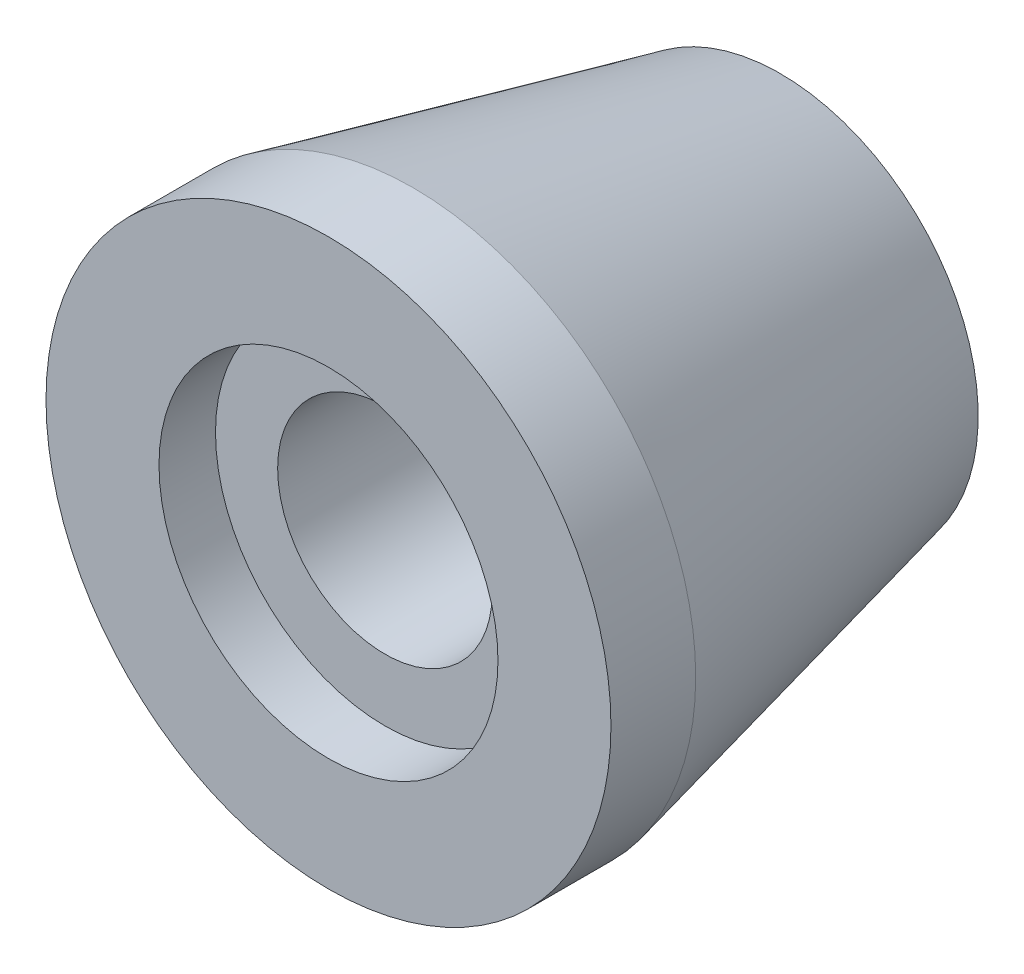
ISO-10303-21;
HEADER;
FILE_DESCRIPTION(('STEP AP214'),'2;1');
FILE_NAME('part.step','',(''),(''),'','','');
FILE_SCHEMA(('AUTOMOTIVE_DESIGN { 1 0 10303 214 1 1 1 1 }'));
ENDSEC;
DATA;
#1=APPLICATION_CONTEXT('core data for automotive mechanical design processes');
#2=APPLICATION_PROTOCOL_DEFINITION('international standard','automotive_design',2000,#1);
#3=PRODUCT_CONTEXT('',#1,'mechanical');
#4=PRODUCT('Part','Part','',(#3));
#5=PRODUCT_RELATED_PRODUCT_CATEGORY('part','',(#4));
#6=PRODUCT_DEFINITION_FORMATION('','',#4);
#7=PRODUCT_DEFINITION_CONTEXT('part definition',#1,'design');
#8=PRODUCT_DEFINITION('design','',#6,#7);
#9=PRODUCT_DEFINITION_SHAPE('','',#8);
#10=(LENGTH_UNIT() NAMED_UNIT(*) SI_UNIT(.MILLI.,.METRE.));
#11=(NAMED_UNIT(*) PLANE_ANGLE_UNIT() SI_UNIT($,.RADIAN.));
#12=(NAMED_UNIT(*) SI_UNIT($,.STERADIAN.) SOLID_ANGLE_UNIT());
#13=UNCERTAINTY_MEASURE_WITH_UNIT(LENGTH_MEASURE(1.E-05),#10,'distance_accuracy_value','');
#14=(GEOMETRIC_REPRESENTATION_CONTEXT(3) GLOBAL_UNCERTAINTY_ASSIGNED_CONTEXT((#13)) GLOBAL_UNIT_ASSIGNED_CONTEXT((#10,
#11,#12)) REPRESENTATION_CONTEXT('',''));
#15=CARTESIAN_POINT('',(0.,0.,0.));
#16=DIRECTION('',(0.,0.,1.));
#17=DIRECTION('',(1.,0.,0.));
#18=AXIS2_PLACEMENT_3D('',#15,#16,#17);
#19=CARTESIAN_POINT('',(0.,7.,0.));
#20=DIRECTION('',(0.,0.,-1.));
#21=DIRECTION('',(-1.,0.,0.));
#22=AXIS2_PLACEMENT_3D('',#19,#20,#21);
#23=PLANE('',#22);
#24=CARTESIAN_POINT('',(0.,0.,0.));
#25=DIRECTION('',(0.,0.,-1.));
#26=DIRECTION('',(-1.,0.,0.));
#27=AXIS2_PLACEMENT_3D('',#24,#25,#26);
#28=CIRCLE('',#27,7.);
#29=CARTESIAN_POINT('',(-7.,0.,0.));
#30=VERTEX_POINT('',#29);
#31=EDGE_CURVE('E70',#30,#30,#28,.T.);
#32=ORIENTED_EDGE('',*,*,#31,.T.);
#33=EDGE_LOOP('',(#32));
#34=FACE_BOUND('',#33,.T.);
#35=CARTESIAN_POINT('',(0.,0.,0.));
#36=DIRECTION('',(0.,0.,-1.));
#37=DIRECTION('',(-1.,0.,0.));
#38=AXIS2_PLACEMENT_3D('',#35,#36,#37);
#39=CIRCLE('',#38,3.8);
#40=CARTESIAN_POINT('',(-3.8,0.,0.));
#41=VERTEX_POINT('',#40);
#42=EDGE_CURVE('E10',#41,#41,#39,.T.);
#43=ORIENTED_EDGE('',*,*,#42,.F.);
#44=EDGE_LOOP('',(#43));
#45=FACE_BOUND('',#44,.T.);
#46=ADVANCED_FACE('F43',(#34,#45),#23,.T.);
#47=CARTESIAN_POINT('',(0.,0.,0.));
#48=DIRECTION('',(0.,0.,-1.));
#49=DIRECTION('',(-1.,0.,0.));
#50=AXIS2_PLACEMENT_3D('',#47,#48,#49);
#51=CYLINDRICAL_SURFACE('',#50,3.8);
#52=ORIENTED_EDGE('',*,*,#42,.T.);
#53=EDGE_LOOP('',(#52));
#54=FACE_BOUND('',#53,.T.);
#55=CARTESIAN_POINT('',(0.,0.,14.));
#56=DIRECTION('',(0.,0.,-1.));
#57=DIRECTION('',(-1.,0.,0.));
#58=AXIS2_PLACEMENT_3D('',#55,#56,#57);
#59=CIRCLE('',#58,3.8);
#60=CARTESIAN_POINT('',(-3.8,0.,14.));
#61=VERTEX_POINT('',#60);
#62=EDGE_CURVE('E47',#61,#61,#59,.T.);
#63=ORIENTED_EDGE('',*,*,#62,.F.);
#64=EDGE_LOOP('',(#63));
#65=FACE_BOUND('',#64,.T.);
#66=ADVANCED_FACE('F88',(#54,#65),#51,.F.);
#67=CARTESIAN_POINT('',(0.,3.8,14.));
#68=DIRECTION('',(0.,0.,1.));
#69=DIRECTION('',(1.,0.,0.));
#70=AXIS2_PLACEMENT_3D('',#67,#68,#69);
#71=PLANE('',#70);
#72=ORIENTED_EDGE('',*,*,#62,.T.);
#73=EDGE_LOOP('',(#72));
#74=FACE_BOUND('',#73,.T.);
#75=CARTESIAN_POINT('',(0.,0.,14.));
#76=DIRECTION('',(0.,0.,-1.));
#77=DIRECTION('',(-1.,0.,0.));
#78=AXIS2_PLACEMENT_3D('',#75,#76,#77);
#79=CIRCLE('',#78,6.);
#80=CARTESIAN_POINT('',(-6.,0.,14.));
#81=VERTEX_POINT('',#80);
#82=EDGE_CURVE('E52',#81,#81,#79,.T.);
#83=ORIENTED_EDGE('',*,*,#82,.F.);
#84=EDGE_LOOP('',(#83));
#85=FACE_BOUND('',#84,.T.);
#86=ADVANCED_FACE('F93',(#74,#85),#71,.T.);
#87=CARTESIAN_POINT('',(0.,0.,0.));
#88=DIRECTION('',(0.,0.,-1.));
#89=DIRECTION('',(-1.,0.,0.));
#90=AXIS2_PLACEMENT_3D('',#87,#88,#89);
#91=CYLINDRICAL_SURFACE('',#90,6.);
#92=ORIENTED_EDGE('',*,*,#82,.T.);
#93=EDGE_LOOP('',(#92));
#94=FACE_BOUND('',#93,.T.);
#95=CARTESIAN_POINT('',(0.,0.,16.));
#96=DIRECTION('',(0.,0.,-1.));
#97=DIRECTION('',(-1.,0.,0.));
#98=AXIS2_PLACEMENT_3D('',#95,#96,#97);
#99=CIRCLE('',#98,6.);
#100=CARTESIAN_POINT('',(-6.,0.,16.));
#101=VERTEX_POINT('',#100);
#102=EDGE_CURVE('E60',#101,#101,#99,.T.);
#103=ORIENTED_EDGE('',*,*,#102,.F.);
#104=EDGE_LOOP('',(#103));
#105=FACE_BOUND('',#104,.T.);
#106=ADVANCED_FACE('F92',(#94,#105),#91,.F.);
#107=CARTESIAN_POINT('',(0.,6.,16.));
#108=DIRECTION('',(0.,0.,1.));
#109=DIRECTION('',(1.,0.,0.));
#110=AXIS2_PLACEMENT_3D('',#107,#108,#109);
#111=PLANE('',#110);
#112=ORIENTED_EDGE('',*,*,#102,.T.);
#113=EDGE_LOOP('',(#112));
#114=FACE_BOUND('',#113,.T.);
#115=CARTESIAN_POINT('',(0.,0.,16.));
#116=DIRECTION('',(0.,0.,-1.));
#117=DIRECTION('',(-1.,0.,0.));
#118=AXIS2_PLACEMENT_3D('',#115,#116,#117);
#119=CIRCLE('',#118,9.99999999999999);
#120=CARTESIAN_POINT('',(-9.99999999999999,0.,16.));
#121=VERTEX_POINT('',#120);
#122=EDGE_CURVE('E65',#121,#121,#119,.T.);
#123=ORIENTED_EDGE('',*,*,#122,.F.);
#124=EDGE_LOOP('',(#123));
#125=FACE_BOUND('',#124,.T.);
#126=ADVANCED_FACE('F84',(#114,#125),#111,.T.);
#127=CARTESIAN_POINT('',(0.,0.,0.));
#128=DIRECTION('',(0.,0.,-1.));
#129=DIRECTION('',(-1.,0.,0.));
#130=AXIS2_PLACEMENT_3D('',#127,#128,#129);
#131=CYLINDRICAL_SURFACE('',#130,9.99999999999999);
#132=ORIENTED_EDGE('',*,*,#122,.T.);
#133=EDGE_LOOP('',(#132));
#134=FACE_BOUND('',#133,.T.);
#135=CARTESIAN_POINT('',(0.,0.,13.));
#136=DIRECTION('',(0.,0.,-1.));
#137=DIRECTION('',(-1.,0.,0.));
#138=AXIS2_PLACEMENT_3D('',#135,#136,#137);
#139=CIRCLE('',#138,9.99999999999999);
#140=CARTESIAN_POINT('',(-9.99999999999999,0.,13.));
#141=VERTEX_POINT('',#140);
#142=EDGE_CURVE('E63',#141,#141,#139,.T.);
#143=ORIENTED_EDGE('',*,*,#142,.F.);
#144=EDGE_LOOP('',(#143));
#145=FACE_BOUND('',#144,.T.);
#146=ADVANCED_FACE('F77',(#134,#145),#131,.T.);
#147=CARTESIAN_POINT('',(0.,0.,0.));
#148=DIRECTION('',(0.,0.,1.));
#149=DIRECTION('',(1.,0.,0.));
#150=AXIS2_PLACEMENT_3D('',#147,#148,#149);
#151=CONICAL_SURFACE('',#150,7.,0.226798848053886);
#152=ORIENTED_EDGE('',*,*,#142,.T.);
#153=EDGE_LOOP('',(#152));
#154=FACE_BOUND('',#153,.T.);
#155=ORIENTED_EDGE('',*,*,#31,.F.);
#156=EDGE_LOOP('',(#155));
#157=FACE_BOUND('',#156,.T.);
#158=ADVANCED_FACE('F74',(#154,#157),#151,.T.);
#159=CLOSED_SHELL('',(#46,#66,#86,#106,#126,#146,#158));
#160=MANIFOLD_SOLID_BREP('B2',#159);
#161=ADVANCED_BREP_SHAPE_REPRESENTATION('',(#18,#160),#14);
#162=SHAPE_DEFINITION_REPRESENTATION(#9,#161);
ENDSEC;
END-ISO-10303-21;
